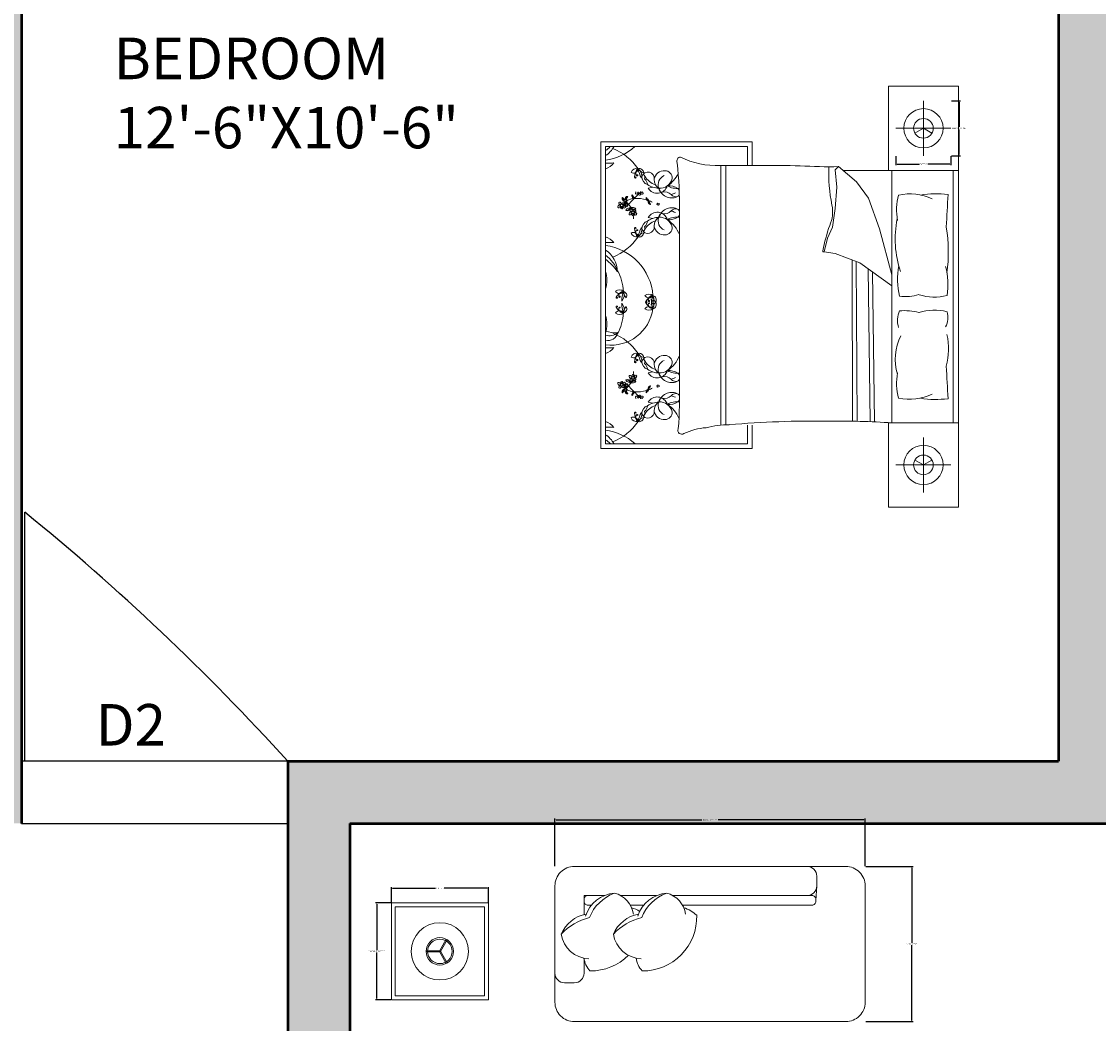
# Model space of a CAD drawing. Units: inches. Extents: x -12 to 604, y -566 to 58.
# Tile 9 of 12: x 280 to 436, y -219 to -74. Entities that reach past the tile are written whole.
import ezdxf

# ---------------------------------------------------------------- set-up
doc = ezdxf.new("R2010")
doc.units = ezdxf.units.IN
doc.header["$MEASUREMENT"] = 0
for name, color, linetype, lineweight in [('A-ANNO-DIMS', 2, 'Continuous', 18), ('A-ANNO-TEXT', 7, 'Continuous', 18), ('A-AREA-IDEN', 7, 'Continuous', 18), ('A-DOOR', 4, 'Continuous', 25), ('A-FURN', 8, 'Continuous', 18), ('A-WALL', 7, 'Continuous', 50), ('A-WALL-PATT', 18, 'Continuous', 13)]:
    doc.layers.add(name, color=color, linetype=linetype, lineweight=lineweight)
doc.styles.get("Standard").update_dxf_attribs({"font": 'arial.ttf'})
doc.dimstyles.get("Standard").update_dxf_attribs({"dimtxt": 0.18, "dimasz": 0.18, "dimexe": 0.18, "dimexo": 0.0625, "dimgap": 0.09, "dimtad": 0, "dimtih": 1, "dimtoh": 1, "dimdec": 0, "dimzin": 0, "dimdsep": 46, "dimlunit": 3, "dimtxsty": 'Standard', "dimcen": 0.09, "dimadec": 0, "dimazin": 0, "dimtfac": 1, "dimtdec": 0, "dimtofl": 0, "dimtmove": 0, "dimatfit": 3, "dimfxl": 1, "dimtolj": 1, "dimtzin": 0, "dimarcsym": 0})

# ---------------------------------------------------------------- blocks, each defined once
blk = doc.blocks.new('DAY BED1')
at = {"color": 0}
blk.add_line((0.3, 0.25), (0.225, 0.2549), dxfattribs=at)
blk.add_lwpolyline([(-0.3, 0, -0.414214), (-0.4, 0.1), (-0.4, 0.1, 0.317837), (-0.4, 0.1, -0.414214), (-0.4, 0.1), (-0.4, 0.1, 1.186185), (-0.4, 0.1, -0.414214), (-0.4, 0.1), (-0.4, 1.5, -0.414214), (-0.3, 1.6), (0.3, 1.6, -0.414214), (0.4, 1.5), (0.4, 0.1, -0.414214), (0.3, 0)], format="xyb", close=True, dxfattribs=at)
for points in [[(-0.0725, 1.45), (-0.15, 1.45, -0.414214), (-0.2, 1.5), (-0.2, 1.55, -0.414214), (-0.15, 1.6)], [(-0.0756, 1.4249, -0.356772), (0.0505, 1.5682, -0.249542), (0.1543, 1.4384, 9.61688)], [(0.0505, 1.5682, -0.14773), (0.1364, 1.422, -0.213343), (0.2624, 1.2931, -0.178662)], [(-0.0725, 1.4501, 0.165541), (-0.1386, 1.4192, 0.200231), (-0.0581, 1.2207, 0.121523)], [(0.25, 1.3448), (0.25, 1.45), (0.1517, 1.45, -0.414214)], [(0.2, 1.4118), (0.2, 1.43, -0.414214), (0.22, 1.45), (0.23, 1.45, -0.414214), (0.25, 1.43)], [(0.1433, 1.4422, -0.306663), (0.2624, 1.2931, -0.30633), (0.1536, 1.1957, 0.872847)], [(0.25, 1.43), (0.25, 1.3448, -0.414214)], [(-0.0756, 1.1556, -0.356772), (0.0505, 1.2988, -0.249542), (0.1543, 1.169, 9.61688)], [(0.0505, 1.2988, -0.14773), (0.1364, 1.1527, -0.213343), (0.2624, 1.0238, -0.178662)], [(0.25, 1.2616), (0.25, 1.0755, -0.414214)], [(-0.0725, 1.1808, 0.165541), (-0.1386, 1.1498, 0.425989), (0.1479, 0.869, 0.121523), (0.1873, 0.9357, -7.115464)], [(0.1433, 1.1729, -0.306663), (0.2624, 1.0238, -0.30633), (0.1536, 0.9263, 0.872847)], [(0.1678, 1.1631, 0.071865), (0.1873, 1.205, -7.115464)], [(0.2, 1.1425), (0.2, 1.2113, -0.414214)], [(0.25, 0.9923), (0.25, 0.2749, -0.414214), (0.23, 0.2549), (0.22, 0.2549, -0.414214), (0.2, 0.2749), (0.2, 0.9419, -0.414214)], [(0.25, 0.3775), (0.25, 0.3, 0.414214), (0.3, 0.25), (0.35, 0.25, 0.414214), (0.4, 0.3)]]:
    blk.add_lwpolyline(points, format="xyb", dxfattribs=at)
for points in [[(0.25, 1.0755), (0.25, 1.2616)], [(0.25, 0.3775), (0.25, 0.9923)]]:
    blk.add_lwpolyline(points, dxfattribs=at)
blk = doc.blocks.new('SIDE-TABLE-WITH-LAMP')
for p, q in [((6.94, 7.06), (7.93, 8.77)), ((7.09, 6.97), (8.08, 8.68)), ((7.01, 7.1), (5.03, 7.1)), ((7.01, 6.92), (5.03, 6.92)), ((6.94, 6.97), (7.93, 5.26)), ((7.09, 7.06), (8.08, 5.34))]:
    blk.add_line(p, q)
at = {"ltscale": 0.03}
blk.add_lwpolyline([(14.03, 14.03), (14.03, 0), (0, 0), (0, 14.03)], close=True, dxfattribs=at)
blk.add_lwpolyline([(13.46, 0.56), (13.46, 13.46), (0.56, 13.46), (0.56, 0.56)], close=True)
for radius in [4.14, 1.98, 1.77]:
    blk.add_circle((7.01, 7.01), radius)
blk = doc.blocks.new('BEDSIDE-LAMP-144')
for p, q in [((3.98, 7.95), (3.98, 0)), ((0, 3.98), (7.95, 3.98))]:
    blk.add_line(p, q)
for points in [[(3.98, 3.98), (2.75, 4.69)], [(3.98, 3.98), (5.21, 4.69)]]:
    blk.add_lwpolyline(points)
for radius in [2.84, 1.42]:
    blk.add_circle((3.98, 3.98), radius)
blk = doc.blocks.new('*D23')
at = {"layer": 'A-ANNO-DIMS', "color": 0, "lineweight": -2, "transparency": 16777216}
for p, q in [((357.47, -196.01), (357.47, -189.16)), ((357.65, -189.34), (378.73, -189.34)), ((402.17, -189.34), (381.1, -189.34)), ((402.35, -196.01), (402.35, -189.16))]:
    blk.add_line(p, q, dxfattribs=at)
at = {"layer": 'A-ANNO-DIMS', "color": 0, "transparency": 16777216}
for points in [[(357.65, -189.31), (357.65, -189.37), (357.47, -189.34)], [(402.17, -189.31), (402.17, -189.37), (402.35, -189.34)]]:
    blk.add_solid(points, dxfattribs=at)
at = {"layer": 'Defpoints', "color": 0, "transparency": 16777216}
for p in [(357.47, -189.34), (357.47, -196.07), (402.35, -196.07)]:
    blk.add_point(p, dxfattribs=at)
at = {"layer": 'A-ANNO-DIMS', "color": 0, "transparency": 16777216, "insert": (379.91, -189.34), "char_height": 0.18, "attachment_point": 5}
blk.add_mtext('\\A1;DAYBED 3\'-9" TYP.', dxfattribs=at)
blk = doc.blocks.new('*D24')
at = {"layer": 'A-ANNO-DIMS', "color": 0, "lineweight": -2, "transparency": 16777216}
for p, q in [((402.42, -196.07), (409.27, -196.07)), ((409.09, -196.25), (409.09, -207.11)), ((409.09, -218.33), (409.09, -207.47)), ((402.42, -218.51), (409.27, -218.51))]:
    blk.add_line(p, q, dxfattribs=at)
at = {"layer": 'A-ANNO-DIMS', "color": 0, "transparency": 16777216}
for points in [[(409.06, -196.25), (409.12, -196.25), (409.09, -196.07)], [(409.06, -218.33), (409.12, -218.33), (409.09, -218.51)]]:
    blk.add_solid(points, dxfattribs=at)
at = {"layer": 'Defpoints', "color": 0, "transparency": 16777216}
for p in [(402.35, -196.07), (409.09, -196.07), (402.35, -218.51)]:
    blk.add_point(p, dxfattribs=at)
at = {"layer": 'A-ANNO-DIMS', "color": 0, "transparency": 16777216, "insert": (409.09, -207.29), "char_height": 0.18, "attachment_point": 5}
blk.add_mtext('\\A1;1\'-10 1/2" TYP.', dxfattribs=at)
blk = doc.blocks.new('*D31')
at = {"layer": 'A-ANNO-DIMS', "color": 0, "lineweight": -2, "transparency": 16777216}
for p, q in [((333.76, -201.33), (331.53, -201.33)), ((331.71, -201.51), (331.71, -208.17)), ((331.71, -215.18), (331.71, -208.53)), ((333.76, -215.36), (331.53, -215.36))]:
    blk.add_line(p, q, dxfattribs=at)
at = {"layer": 'A-ANNO-DIMS', "color": 0, "transparency": 16777216}
for points in [[(331.68, -201.51), (331.74, -201.51), (331.71, -201.33)], [(331.68, -215.18), (331.74, -215.18), (331.71, -215.36)]]:
    blk.add_solid(points, dxfattribs=at)
at = {"layer": 'Defpoints', "color": 0, "transparency": 16777216}
for p in [(331.71, -201.33), (333.82, -201.33), (333.82, -215.36)]:
    blk.add_point(p, dxfattribs=at)
at = {"layer": 'A-ANNO-DIMS', "color": 0, "transparency": 16777216, "insert": (331.71, -208.35), "char_height": 0.18, "attachment_point": 5}
blk.add_mtext('\\A1;END TABLE 1\'-2" TYP.', dxfattribs=at)
blk = doc.blocks.new('*D32')
at = {"layer": 'A-ANNO-DIMS', "color": 0, "lineweight": -2, "transparency": 16777216}
for p, q in [((333.82, -201.27), (333.82, -199.05)), ((334, -199.23), (340.2, -199.23)), ((347.66, -199.23), (341.46, -199.23)), ((347.84, -201.27), (347.84, -199.05))]:
    blk.add_line(p, q, dxfattribs=at)
at = {"layer": 'A-ANNO-DIMS', "color": 0, "transparency": 16777216}
for points in [[(334, -199.2), (334, -199.26), (333.82, -199.23)], [(347.66, -199.2), (347.66, -199.26), (347.84, -199.23)]]:
    blk.add_solid(points, dxfattribs=at)
at = {"layer": 'Defpoints', "color": 0, "transparency": 16777216}
for p in [(347.84, -199.23), (333.82, -201.33), (347.84, -201.33)]:
    blk.add_point(p, dxfattribs=at)
at = {"layer": 'A-ANNO-DIMS', "color": 0, "transparency": 16777216, "insert": (340.83, -199.23), "char_height": 0.18, "attachment_point": 5}
blk.add_mtext('\\A1;1\'-2" TYP.', dxfattribs=at)
blk = doc.blocks.new('*D41')
at = {"layer": 'A-ANNO-DIMS', "color": 0, "lineweight": -2, "transparency": 16777216}
for p, q in [((414.81, -85.35), (416.12, -85.35)), ((415.94, -85.53), (415.94, -89.14)), ((415.94, -93.12), (415.94, -89.51)), ((414.81, -93.3), (416.12, -93.3))]:
    blk.add_line(p, q, dxfattribs=at)
at = {"layer": 'A-ANNO-DIMS', "color": 0, "transparency": 16777216}
for points in [[(415.91, -85.53), (415.97, -85.53), (415.94, -85.35)], [(415.91, -93.12), (415.97, -93.12), (415.94, -93.3)]]:
    blk.add_solid(points, dxfattribs=at)
at = {"layer": 'Defpoints', "color": 0, "transparency": 16777216}
for p in [(414.75, -85.35), (414.75, -93.3), (415.94, -93.3)]:
    blk.add_point(p, dxfattribs=at)
at = {"layer": 'A-ANNO-DIMS', "color": 0, "transparency": 16777216, "insert": (415.94, -89.33), "char_height": 0.18, "attachment_point": 5}
blk.add_mtext('\\A1;LAMP C 0\'-8" TYP.', dxfattribs=at)
blk = doc.blocks.new('*D42')
at = {"layer": 'A-ANNO-DIMS', "color": 0, "lineweight": -2, "transparency": 16777216}
for p, q in [((406.79, -93.37), (406.79, -94.68)), ((414.75, -93.37), (414.75, -94.68)), ((406.97, -94.5), (410.13, -94.5)), ((414.57, -94.5), (411.41, -94.5))]:
    blk.add_line(p, q, dxfattribs=at)
at = {"layer": 'A-ANNO-DIMS', "color": 0, "transparency": 16777216}
for points in [[(406.97, -94.47), (406.97, -94.53), (406.79, -94.5)], [(414.57, -94.47), (414.57, -94.53), (414.75, -94.5)]]:
    blk.add_solid(points, dxfattribs=at)
at = {"layer": 'Defpoints', "color": 0, "transparency": 16777216}
for p in [(406.79, -93.3), (414.75, -93.3), (406.79, -94.5)]:
    blk.add_point(p, dxfattribs=at)
at = {"layer": 'A-ANNO-DIMS', "color": 0, "transparency": 16777216, "insert": (410.77, -94.5), "char_height": 0.18, "attachment_point": 5}
blk.add_mtext('\\A1;0\'-8" TYP.', dxfattribs=at)

msp = doc.modelspace()

# ---------------------------------------------------------------- hatches: boundary and pattern name
at = {"layer": 'A-WALL-PATT'}
h = msp.add_hatch(color=256, dxfattribs=at)
h.dxf.hatch_style = 1
h.paths.add_polyline_path([(169.32, 11.14), (169.32, 17.14), (160.32, 17.14), (160.32, 11.14), (118.32, 11.14), (118.32, 6.64), (118.32, 2.14), (127.32, 2.14), (169.32, 2.14)])
h.paths.add_polyline_path([(127.32, -13.61), (118.32, -13.61), (118.32, -29.36), (34.82, -29.36), (24.32, -29.36), (24.32, -38.36), (39.32, -38.36), (118.32, -38.36), (118.32, -126.86), (127.32, -126.86), (127.32, -117.86)])
h.paths.add_polyline_path([(82.32, -92.36), (39.32, -92.36), (39.32, -56.22), (30.32, -56.22), (24.32, -56.22), (24.32, -65.22), (30.32, -65.22), (30.32, -113.36), (24.32, -113.36), (24.32, -122.36), (39.32, -122.36), (39.32, -101.36), (82.32, -101.36), (82.32, -96.86)], flags=17)
h.paths.add_polyline_path([(280.32, 11.14), (238.32, 11.14), (238.32, 17.14), (229.32, 17.14), (229.32, 12.64), (229.32, 11.14), (229.32, 2.14), (271.32, 2.14), (271.32, -117.86), (163.32, -117.86), (163.32, -126.86), (271.32, -126.86), (271.32, -189.86), (280.32, -189.86), (280.32, -180.86)])
h.paths.add_polyline_path([(415.32, 17.14), (406.32, 17.14), (406.32, 11.14), (358.32, 11.14), (358.32, -21.86), (367.32, -21.86), (367.32, 2.14), (415.32, 2.14)], flags=17)
h.paths.add_polyline_path([(484.55, -45.86), (448.32, -45.86), (448.32, 2.14), (448.32, 17.14), (439.32, 17.14), (439.32, 12.64), (439.32, 2.14), (439.32, -45.86), (367.32, -45.86), (358.32, -45.86), (358.32, -54.86), (430.32, -54.86), (430.32, -69.59), (430.32, -180.86), (318.82, -180.86), (318.82, -189.86), (318.82, -331.86), (327.82, -331.86), (327.82, -189.86), (439.32, -189.86), (439.32, -180.86), (439.32, -54.86), (483.5, -54.86), (484.55, -54.86)])
h.paths.add_polyline_path([(529.32, 11.14), (481.32, 11.14), (481.32, 17.14), (472.32, 17.14), (472.32, 12.64), (472.32, 2.14), (520.32, 2.14), (520.32, -21.86), (529.32, -21.86)])
h.paths.add_polyline_path([(598.32, -45.86), (582.42, -45.86), (582.42, -50.36), (582.42, -54.86), (589.32, -54.86), (589.32, -99.86), (598.32, -99.86), (604.32, -99.86), (604.32, -90.86), (598.32, -90.86)])
h.paths.add_polyline_path([(598.32, -168.86), (604.32, -168.86), (604.32, -159.86), (589.32, -159.86), (589.32, -180.86), (477.32, -180.86), (477.32, -189.86), (477.32, -259.86), (486.32, -259.86), (486.32, -189.86), (589.32, -189.86), (589.32, -204.86), (598.32, -204.86), (604.32, -204.86), (604.32, -195.86), (598.32, -195.86)])
h.paths.add_polyline_path([(598.32, -244.86), (604.32, -244.86), (604.32, -235.86), (598.32, -235.86), (589.32, -235.86), (589.32, -250.86), (522.32, -250.86), (522.32, -259.86), (589.32, -259.86), (589.32, -274.86), (598.32, -274.86), (604.32, -274.86), (604.32, -265.86), (598.32, -265.86)])
h.paths.add_polyline_path([(598.32, -333.28), (604.32, -333.28), (604.32, -324.28), (598.32, -324.28), (598.32, -321.87), (598.32, -318.28), (604.32, -318.28), (604.32, -309.28), (598.32, -309.28), (589.32, -309.28), (589.32, -341.95), (589.38, -341.95), (589.38, -363.16), (589.32, -381.86), (565.32, -381.86), (565.32, -390.86), (589.32, -390.86), (589.32, -450.86), (598.32, -450.86), (604.32, -450.86), (604.32, -441.86), (598.32, -441.86), (598.32, -390.86), (604.32, -390.86), (604.32, -381.86), (598.32, -381.86)])
h.paths.add_polyline_path([(541.32, -345.86), (424.32, -345.86), (424.32, -354.86), (532.32, -354.86), (532.32, -474.86), (463.39, -474.86), (463.39, -483.86), (553.32, -483.86), (553.32, -474.86), (541.32, -474.86), (541.32, -390.86), (541.32, -381.86)])
h.paths.add_polyline_path([(604.32, -474.86), (589.32, -474.86), (553.32, -474.86), (553.32, -483.86), (598.32, -483.86), (604.32, -483.86)])
h.paths.add_polyline_path([(388.32, -483.86), (388.32, -474.86), (388.32, -460.13), (388.32, -333.86), (388.32, -322.86), (379.32, -322.86), (379.32, -331.86), (379.32, -333.86), (379.32, -474.86), (379.32, -520.86), (344.32, -520.86), (344.32, -529.86), (379.32, -529.86), (388.32, -529.86)])
h.paths.add_polyline_path([(284.32, -520.86), (249.32, -520.86), (249.32, -474.86), (249.32, -368.36), (240.32, -368.36), (240.32, -474.86), (238.52, -474.86), (238.52, -483.86), (240.32, -483.86), (240.32, -529.86), (249.32, -529.86), (284.32, -529.86)])
h.paths.add_polyline_path([(178.82, -474.86), (158.91, -474.86), (158.91, -483.86), (162.32, -483.86), (178.82, -483.86)])
h.paths.add_polyline_path([(84.32, -474.86), (84.32, -366.86), (75.32, -366.86), (75.32, -474.86), (39.32, -474.86), (39.32, -453.86), (24.32, -453.86), (24.32, -462.86), (30.32, -462.86), (30.32, -483.86), (84.32, -483.86)])
h.paths.add_polyline_path([(39.32, -342.86), (75.32, -342.86), (84.32, -342.86), (179.67, -342.86), (179.67, -333.86), (39.32, -333.86), (39.32, -318.86), (24.32, -318.86), (24.32, -327.86), (30.32, -327.86), (30.32, -432.86), (24.32, -432.86), (24.32, -441.86), (30.32, -441.86), (39.32, -441.86)])
h.paths.add_polyline_path([(249.32, -252.86), (115.32, -252.86), (115.32, -225.86), (106.32, -225.86), (106.32, -252.86), (39.32, -252.86), (39.32, -237.86), (24.32, -237.86), (24.32, -246.86), (30.32, -246.86), (30.32, -267.86), (24.32, -267.86), (24.32, -276.86), (39.32, -276.86), (39.32, -261.86), (240.32, -261.86), (240.32, -331.86), (249.32, -331.86), (266.82, -331.86), (266.82, -322.86), (249.32, -322.86)])
h.paths.add_polyline_path([(127.32, -180.86), (39.32, -180.86), (24.32, -180.86), (24.32, -189.86), (39.32, -189.86), (127.32, -189.86)])
h.paths.add_polyline_path([(39.32, -159.86), (24.32, -159.86), (24.32, -168.86), (30.32, -168.86), (30.32, -180.86), (39.32, -180.86)])
h.paths.add_polyline_path([(470.51, -17.27), (512.48, -17.27), (512.48, 5.12), (470.51, 5.12)], flags=9)
h.paths.add_polyline_path([(484.21, -244.26), (526.45, -244.26), (526.45, -221.87), (484.21, -221.87)], flags=24)
h.paths.add_polyline_path([(36.91, -442.88), (83.54, -442.88), (83.54, -420.5), (36.91, -420.5)], flags=25)

# ---------------------------------------------------------------- linework, layer by layer
at = {"layer": 'A-DOOR'}
for p, q in [((280.8, -180.86), (280.8, -144.86)), ((318.82, -180.86), (280.32, -180.86)), ((280.32, -180.86), (280.32, -189.86)), ((318.82, -189.86), (318.82, -180.86)), ((280.32, -189.86), (318.82, -189.86))]:
    msp.add_line(p, q, dxfattribs=at)
msp.add_arc((63.22, -412.75), 345.12, 42.2146, 50.9159, dxfattribs=at)
at = {"layer": 'A-FURN'}
for p, q in [((415.84, -83.24), (415.84, -144.1)), ((364.09, -91.27), (386.01, -91.27)), ((364.09, -135.64), (364.09, -91.27)), ((386.01, -91.27), (386.01, -94.72)), ((364.79, -91.98), (364.79, -134.94)), ((385.3, -91.98), (364.79, -91.98)), ((385.3, -94.72), (385.3, -91.98)), ((381.46, -132.26), (381.46, -94.71)), ((382.21, -132.2), (382.21, -94.71)), ((398.01, -95.36), (398.5, -94.87)), ((398.5, -94.87), (401.09, -97.09)), ((398.26, -97.83), (398.01, -95.36)), ((415.84, -95.41), (399.14, -95.41)), ((406.22, -95.41), (406.22, -131.93)), ((415.06, -131.93), (415.06, -95.41)), ((370.96, -97.98), (371.65, -97.84)), ((398.01, -100.91), (398.26, -97.83)), ((401.09, -97.09), (402.81, -99.43)), ((402.81, -99.43), (404.42, -103.87)), ((397.64, -103.62), (398.01, -100.91)), ((370.96, -102.23), (371.65, -102.36)), ((375.48, -126.02), (375.48, -101.32)), ((396.9, -105.22), (397.64, -103.62)), ((404.42, -103.87), (406.22, -110.5)), ((396.41, -107.19), (396.9, -105.22)), ((398.01, -107.44), (396.41, -107.19)), ((401.58, -108.8), (398.01, -107.44)), ((400.53, -131.71), (400.44, -108.36)), ((401.16, -131.71), (401.06, -108.6)), ((406.22, -112.13), (401.58, -108.8)), ((403.07, -131.74), (402.76, -109.64)), ((403.7, -131.76), (403.39, -110.1)), ((370.96, -124.69), (371.65, -124.55)), ((370.96, -128.94), (371.65, -129.07)), ((385.3, -134.94), (385.3, -132.25)), ((386.01, -132.27), (386.01, -135.64)), ((364.79, -134.94), (385.3, -134.94)), ((386.01, -135.64), (364.09, -135.64))]:
    msp.add_line(p, q, dxfattribs=at)
for points in [[(405.7, -95.41), (405.7, -83.24), (415.84, -83.24)], [(415.84, -131.93), (405.7, -131.93), (405.7, -144.1), (415.84, -144.1)]]:
    msp.add_lwpolyline(points, dxfattribs=at)
for points in [[(392.93, -94.74, 0.001242), (381.38, -94.71, -0.127202), (375.63, -93.49)], [(414.33, -98.91, 0.074897), (410.35, -98.98, -0.472817)], [(410.13, -113.39, 0.14099), (414.18, -113.51, 0.235245)], [(410.13, -115.98, -0.14099), (414.18, -115.86, -0.235245)], [(414.33, -128.43, -0.074897), (410.35, -128.36, 0.472817)], [(382.69, -132.19, 0.056112), (379.34, -132.63, 0.095341), (376.12, -133.48)]]:
    msp.add_lwpolyline(points, format="xyb", dxfattribs=at)
for centre in [(367.12, -100.48), (368.76, -101.49), (368.76, -125.42), (367.12, -126.44)]:
    msp.add_circle(centre, 0.155, dxfattribs=at)
for centre, radius, start, end in [((361.94, -88.66), 4.83, 306.3036, 316.4814), ((362.66, -90.05), 3.87, 303.4617, 330.1116), ((363.72, -86.06), 7.95, 277.745, 311.8856), ((362.94, -99.66), 7.95, 34.3865, 68.5908), ((363.55, -92.22), 3.23, 292.5547, 318.9546), ((365.29, -83.37), 11, 267.4081, 273.6519), ((375.67, -94.05), 0.562, 93.98, 207.3412), ((312.13, -100.59), 63.35, 359.3433, 5.6887), ((396.99, -39.07), 55.82, 265.8294, 271.553), ((420.05, -95.91), 22.97, 177.4519, 191.3392), ((369.31, -96.03), 0.881, 77.7115, 159.0387), ((368.83, -95.15), 0.664, 238.4633, 358.2869), ((371.01, -96.49), 2.01, 138.8402, 177.9352), ((369.1, -96.43), 0.0987, 177.9352, 11.4834), ((369.15, -96.42), 0.0479, 11.4834, 127.9409), ((369.8, -95.75), 0.65, 117.6827, 223.7762), ((369.39, -96.14), 0.086, 223.7762, 159.7183), ((369.65, -95.81), 0.659, 2.9516, 103.728), ((374.92, -93.97), 5.56, 192.5173, 207.1824), ((368.76, -96.19), 1.26, 345.4653, 54.2343), ((370.65, -94.46), 1.36, 211.3827, 255.2969), ((370.91, -96.58), 0.913, 350.264, 160.8688), ((371.19, -96.37), 1.14, 175.969, 254.3045), ((369.92, -96.4), 0.56, 333.9755, 53.2681), ((372.92, -94.77), 2.87, 211.2614, 251.7045), ((373.26, -96.92), 1.45, 84.9449, 172.8857), ((373.81, -97.49), 1.41, 111.5819, 201.4221), ((373.4, -96.5), 1.03, 354.4856, 91.0538), ((371.19, -93.82), 4.61, 303.6671, 333.2997), ((369.67, -97.59), 1.21, 6.1662, 51.5825), ((372.69, -94.75), 3.27, 236.2883, 266.5076), ((372.27, -97.22), 1.51, 209.9085, 343.1337), ((373.58, -96.67), 1.77, 182.3591, 234.0401), ((372.64, -96.18), 1.83, 265.2933, 346.921), ((372.91, -98.18), 0.378, 167.3041, 285.1471), ((373.93, -99.99), 2.35, 122.7011, 126.3445), ((374.37, -97.46), 1.94, 199.2822, 299.1751), ((375.03, -95.5), 2.52, 238.8218, 279.1554), ((373.93, -99.99), 2.35, 55.785, 94.7304), ((374.8, -98.63), 0.733, 30.0293, 52.325), ((367.35, -99.48), 0.173, 124.3538, 214.3923), ((367.6, -99.5), 0.403, 190.3057, 287.1958), ((367.72, -99.36), 0.468, 176.9701, 248.2913), ((371.06, -96.89), 4.53, 212.6784, 216.3746), ((367.56, -99.47), 0.179, 216.3746, 291.7548), ((367.99, -99.6), 0.403, 122.8155, 187.3992), ((367.68, -99.76), 0.135, 289.3605, 111.7548), ((367.78, -99.76), 0.135, 221.8703, 44.2646), ((368.17, -99.65), 0.468, 109.4799, 177.6828), ((367.92, -99.35), 0.173, 56.8636, 146.9021), ((368, -99.54), 0.179, 148.8844, 224.2646), ((371.73, -101.79), 4.53, 145.1882, 148.8844), ((369.15, -101.99), 2.53, 94.756, 119.2041), ((374.53, -105.62), 8.32, 132.2412, 142.1744), ((370.33, -99.01), 1.72, 178.3264, 187.1302), ((368.48, -99.24), 0.32, 11.3256, 64.4621), ((369.56, -98.78), 0.962, 190.2588, 210.656), ((368.92, -99.18), 0.292, 188.3432, 274.2869), ((369.17, -99.01), 0.51, 210.656, 242.6341), ((369.56, -98.58), 0.978, 218.2101, 226.3071), ((368.83, -99.4), 0.124, 325.7657, 67.4417), ((364.99, -95.25), 5.78, 313.1541, 322.0459), ((369.27, -104.5), 5.04, 73.5842, 93.8277), ((369.23, -98.72), 0.119, 142.4737, 265.053), ((369.39, -98.7), 0.256, 127.7621, 169.0403), ((369.26, -98.48), 0.36, 265.053, 338.3618), ((369.73, -98.98), 0.471, 113.4276, 137.6104), ((369.68, -98.49), 0.155, 183.2768, 356.7232), ((369.79, -98.77), 0.254, 139.7889, 227.6792), ((369.71, -98.86), 0.134, 227.6792, 350.3487), ((369.19, -98.77), 0.507, 353.0852, 15.7171), ((369.53, -98.83), 0.32, 350.3487, 43.6538), ((370.12, -98.5), 0.373, 198.7263, 262.5032), ((369.82, -98.67), 0.148, 1.1081, 91.8675), ((370.1, -98.75), 0.12, 255.2356, 54.9248), ((369.92, -98.7), 0.258, 11.5637, 52.6358), ((372.38, -99.37), 1.72, 178.3264, 187.1302), ((370.52, -99.61), 0.32, 11.3256, 64.4621), ((371.61, -99.15), 0.962, 190.2588, 210.656), ((370.96, -99.54), 0.292, 188.3432, 274.2869), ((371.22, -99.38), 0.51, 210.656, 242.6341), ((371.61, -98.94), 0.978, 218.2101, 226.3071), ((370.88, -99.76), 0.124, 325.7657, 67.4417), ((373.33, -99.75), 1.25, 41.5653, 105.1471), ((374.02, -97.16), 1.75, 277.436, 299.9149), ((374.95, -98.32), 0.911, 221.5653, 293.8354), ((374.8, -98.63), 0.733, 314.4517, 333.558), ((415.04, -101.08), 8.16, 165.1039, 191.0369), ((408.75, -106.66), 7.84, 65.1316, 101.7583), ((993.48, -132.45), 580.12, 176.68521, 177.14978), ((366.68, -100.71), 0.119, 142.4737, 265.053), ((366.84, -100.69), 0.256, 61.2196, 169.0403), ((366.7, -100.47), 0.36, 265.053, 338.3618), ((367.01, -100.16), 0.306, 157.4086, 261.4386), ((366.83, -100.15), 0.154, 58.0499, 135.6268), ((367.18, -100.97), 0.471, 113.4276, 137.6104), ((366.99, -100.25), 0.103, 172.906, 277.132), ((366.66, -100.44), 0.489, 14.7558, 58.0499), ((367.24, -100.76), 0.254, 139.7889, 227.6792), ((367.16, -100.85), 0.134, 227.6792, 350.3487), ((367.34, -100.31), 0.211, 36.1046, 181.4281), ((366.64, -100.76), 0.507, 353.0852, 15.7171), ((366.97, -100.82), 0.32, 350.3487, 43.6538), ((367.57, -100.49), 0.373, 198.7263, 262.5032), ((367.22, -100.14), 0.213, 270.0645, 331.1507), ((367.4, -100.19), 0.244, 221.8413, 265.7877), ((367.27, -100.66), 0.148, 1.1081, 91.8675), ((367.4, -100.28), 0.152, 263.7526, 41.7054), ((367.36, -100.69), 0.258, 11.5637, 86.365), ((369.15, -101.99), 2.53, 124.0033, 132.4917), ((367.55, -100.74), 0.12, 255.2356, 54.9248), ((366.55, -102.3), 2.7, 63.7819, 68.2913), ((367.99, -100.23), 0.429, 128.3208, 208.8162), ((368.07, -100.2), 0.513, 207.7043, 254.3516), ((368.39, -100.16), 0.706, 157.2305, 229.0635), ((368.15, -99.92), 0.416, 174.4544, 220.6188), ((367.73, -100.49), 0.706, 270.278, 342.111), ((368.2, -101.37), 0.5, 98.7227, 159.3375), ((367.95, -100.73), 0.513, 244.9899, 291.6373), ((365.79, -102.25), 3.03, 30.544, 49.818), ((367.46, -100.52), 0.5, 340.0041, 40.6188), ((368.07, -100.47), 0.416, 278.7227, 324.8872), ((367.99, -100.81), 0.429, 290.5253, 358.5375), ((368.64, -101.18), 0.306, 157.4086, 261.4386), ((368.47, -101.17), 0.154, 58.0499, 135.6268), ((368.83, -100.68), 0.429, 182.8499, 266.1226), ((368.66, -100.38), 0.416, 231.7607, 277.9252), ((368.99, -100.31), 0.706, 214.5369, 286.3699), ((368.29, -101.45), 0.489, 14.7558, 58.0499), ((365.79, -102.25), 3.03, 23.0501, 23.8477), ((368.79, -101.29), 0.5, 37.3105, 97.9252), ((368.97, -101.32), 0.211, 36.1046, 181.4281), ((368.85, -100.6), 0.513, 265.0106, 311.658), ((369.03, -101.3), 0.152, 263.7526, 41.7054), ((371.23, -99.99), 0.292, 147.5332, 233.4768), ((371.49, -99.84), 0.51, 179.1859, 211.164), ((371, -99.95), 0.124, 354.3784, 96.0543), ((369.27, -104.5), 5.04, 63.0032, 69.8941), ((371.88, -99.6), 0.962, 211.164, 231.5612), ((372.05, -98.82), 1.72, 234.6898, 243.4936), ((372.06, -99.7), 0.978, 195.5129, 203.6099), ((370.96, -100.34), 0.32, 357.3579, 50.4944), ((372.34, -100.28), 0.117, 12.7051, 190.4384), ((372.41, -100.26), 0.191, 190.4384, 10.4136), ((374.37, -102.75), 1.94, 60.8249, 160.7178), ((374.95, -101.89), 0.911, 66.1646, 138.4347), ((374.8, -101.58), 0.733, 23.229, 45.5483), ((392.68, -101.4), 4.95, 336.2616, 11.3392), ((368.31, -101.73), 0.119, 142.4737, 265.053), ((368.47, -101.7), 0.256, 61.2196, 169.0403), ((368.33, -101.49), 0.36, 265.053, 338.3618), ((368.81, -101.98), 0.471, 113.4276, 137.6104), ((368.63, -101.26), 0.103, 172.906, 277.132), ((368.87, -101.77), 0.254, 139.7889, 227.6792), ((368.79, -101.86), 0.134, 227.6792, 350.3487), ((368.27, -101.77), 0.507, 353.0852, 15.7171), ((365.79, -102.25), 3.03, 357.1071, 4.7585), ((368.61, -101.83), 0.32, 350.3487, 43.6538), ((368.85, -101.16), 0.213, 270.0645, 331.1507), ((369.03, -101.21), 0.244, 221.8413, 265.7877), ((369.2, -101.5), 0.373, 198.7263, 262.5032), ((368.9, -101.67), 0.148, 1.1081, 91.8675), ((369, -101.71), 0.258, 11.5637, 86.365), ((369.18, -101.75), 0.12, 255.2356, 54.9248), ((371.19, -103.84), 1.14, 105.6955, 184.031), ((369.67, -102.61), 1.21, 308.4175, 353.8338), ((372.92, -105.43), 2.87, 108.2955, 148.7386), ((372.69, -105.46), 3.27, 93.4924, 123.7117), ((372.27, -102.98), 1.51, 16.8663, 150.0915), ((373.58, -103.54), 1.77, 125.9599, 177.6409), ((373.81, -102.72), 1.41, 158.5779, 248.4181), ((372.64, -104.02), 1.83, 13.079, 94.7067), ((372.91, -102.03), 0.378, 74.8529, 192.6959), ((373.93, -100.22), 2.35, 233.6555, 237.2989), ((373.33, -100.46), 1.25, 254.8529, 318.4347), ((375.03, -104.7), 2.52, 79.7133, 121.1782), ((373.93, -100.22), 2.35, 265.2696, 304.215), ((371.19, -106.39), 4.61, 21.4941, 56.3329), ((374.02, -103.04), 1.75, 60.0851, 82.564), ((374.8, -101.58), 0.733, 307.675, 336.7144), ((420.83, -105.37), 14.15, 168.0397, 199.2615), ((369.1, -103.78), 0.0987, 348.5166, 182.0648), ((371.01, -103.71), 2.01, 182.0648, 221.1598), ((369.15, -103.79), 0.0479, 232.0591, 348.5166), ((369.8, -104.46), 0.65, 136.2238, 242.3173), ((369.42, -104.08), 0.0518, 200.2667, 136.2271), ((368.76, -104.02), 1.26, 305.7657, 14.5347), ((374.92, -106.24), 5.56, 152.8176, 167.4827), ((370.91, -103.62), 0.913, 199.1312, 9.736), ((369.92, -103.81), 0.56, 306.7319, 26.0245), ((373.26, -103.29), 1.45, 187.1143, 275.0551), ((373.4, -103.71), 1.03, 268.9462, 5.5144), ((419.41, -111.42), 23.6, 160.1194, 169.3383), ((392.3, -107.25), 22.07, 352.2196, 9.497), ((363.55, -107.99), 3.23, 41.0454, 67.4453), ((365.29, -116.84), 11, 86.3481, 92.5919), ((362.94, -100.55), 7.95, 291.4092, 325.6135), ((368.83, -105.06), 0.664, 1.7131, 121.5367), ((369.31, -104.17), 0.881, 200.9613, 282.2885), ((369.65, -104.4), 0.659, 256.272, 357.0484), ((370.65, -105.74), 1.36, 104.7031, 148.6173), ((363.72, -114.14), 7.95, 4.4623, 82.255), ((362.66, -110.16), 3.87, 1.272, 56.5383), ((396.36, -107.06), 0.147, 178.8623, 289.7536), ((361.94, -111.55), 4.83, 17.8504, 53.6964), ((360.58, -114.09), 7.18, 34.0123, 54.053), ((360.61, -111.31), 4.37, 343.5431, 17.0202), ((359.47, -113.54), 7.95, 4.4623, 27.4146), ((417.75, -111.1), 10.73, 169.8617, 193.6238), ((403.46, -111.91), 10.84, 351.5249, 13.96), ((358.36, -113.04), 6.46, 4.3787, 5.6357), ((353.93, -116.45), 11.55, 19.7217, 19.9028), ((366.8, -113.57), 0.881, 47.7873, 129.1145), ((366.82, -112.57), 0.664, 208.5391, 328.3627), ((368.04, -114.82), 2.01, 108.9159, 148.011), ((367.36, -113.57), 0.65, 87.7585, 193.852), ((366.81, -113.7), 0.086, 193.852, 129.9245), ((372.69, -114.58), 5.56, 162.593, 177.2582), ((366.24, -113.43), 1.26, 315.5411, 24.3101), ((368.74, -112.88), 1.36, 181.4585, 225.3727), ((367.2, -113.55), 0.659, 333.0274, 73.8037), ((371.05, -114.18), 0.881, 47.7873, 129.1145), ((371.08, -113.18), 0.664, 208.5391, 328.3627), ((372.3, -115.43), 2.01, 108.9159, 148.011), ((371.62, -114.17), 0.65, 87.7585, 193.852), ((370.5, -114.04), 1.26, 315.5411, 24.3101), ((376.95, -115.19), 5.56, 162.593, 177.2582), ((371.46, -114.16), 0.659, 333.0274, 73.8037), ((373, -113.49), 1.36, 181.4585, 225.3727), ((408.09, -106.21), 7.46, 264.0129, 285.8293), ((366.42, -113.81), 0.0987, 148.011, 341.5592), ((366.42, -115.14), 0.0987, 18.4408, 211.989), ((368.04, -114.13), 2.01, 211.989, 251.0841), ((366.47, -113.82), 0.0479, 341.5592, 98.0167), ((366.47, -115.12), 0.0479, 261.9833, 18.4408), ((367.36, -115.38), 0.65, 166.148, 272.2415), ((366.85, -115.24), 0.0518, 230.1909, 166.0209), ((372.69, -114.36), 5.56, 182.7418, 197.407), ((366.24, -115.51), 1.26, 335.6899, 44.4589), ((368.74, -116.06), 1.36, 134.6273, 178.5415), ((367.2, -115.4), 0.659, 286.1963, 26.9726), ((371.08, -115.77), 0.664, 31.6373, 151.4609), ((370.68, -114.41), 0.0987, 148.011, 341.5592), ((370.68, -114.53), 0.0987, 18.4408, 211.989), ((372.3, -113.52), 2.01, 211.989, 251.0841), ((370.72, -114.43), 0.0479, 341.5592, 98.0167), ((370.72, -114.51), 0.0479, 261.9833, 18.4408), ((371.62, -114.77), 0.65, 166.148, 272.2415), ((371.07, -114.31), 0.086, 193.852, 129.9245), ((371.1, -114.63), 0.0518, 230.1909, 166.0209), ((370.5, -114.9), 1.26, 335.6899, 44.4589), ((376.95, -113.76), 5.56, 182.7418, 197.407), ((371.46, -114.79), 0.659, 286.1963, 26.9726), ((373, -115.45), 1.36, 134.6273, 178.5415), ((365.56, -114.54), 6.15, 262.8636, 351.8197), ((360.61, -117.63), 4.37, 342.9798, 16.4569), ((358.36, -115.9), 6.46, 354.3643, 355.6213), ((353.93, -112.5), 11.55, 340.0972, 340.2783), ((366.82, -116.38), 0.664, 31.6373, 151.4609), ((366.8, -115.38), 0.881, 230.8855, 312.2127), ((359.47, -115.41), 7.95, 332.5854, 355.5377), ((371.05, -114.77), 0.881, 230.8855, 312.2127), ((410.24, -117.1), 3.23, 155.0183, 198.5407), ((408.09, -123.16), 7.46, 74.1707, 95.9871), ((411.29, -116.7), 3.01, 333.3437, 16.1026), ((366.12, -115.34), 3.56, 248.117, 276.6195), ((365.13, -118.6), 1.43, 256.3898, 349.0739), ((365.32, -117.53), 1.8, 252.8609, 311.9049), ((362.94, -126.37), 7.95, 34.3865, 68.5908), ((414.44, -122.74), 7.75, 153.8761, 196.1746), ((403.68, -121.21), 10.7, 346.3427, 11.1841), ((365.29, -110.08), 11, 267.4081, 273.6519), ((363.55, -118.93), 3.23, 292.5547, 318.9546), ((369.31, -122.74), 0.881, 77.7115, 159.0387), ((368.83, -121.86), 0.664, 238.4633, 358.2869), ((371.01, -123.2), 2.01, 138.8402, 177.9352), ((369.8, -122.46), 0.65, 117.6827, 223.7762), ((369.39, -122.85), 0.086, 223.7762, 159.7183), ((369.65, -122.52), 0.659, 2.9516, 103.728), ((370.65, -121.17), 1.36, 211.3827, 255.2969), ((368.76, -122.9), 1.26, 345.4653, 54.2343), ((374.92, -120.68), 5.56, 192.5173, 207.1824), ((370.91, -123.29), 0.913, 350.264, 160.8688), ((371.19, -123.08), 1.14, 175.969, 254.3045), ((369.92, -123.11), 0.56, 333.9755, 53.2681), ((372.92, -121.48), 2.87, 211.2614, 251.7045), ((373.26, -123.63), 1.45, 84.9449, 172.8857), ((373.81, -124.2), 1.41, 111.5819, 201.4221), ((373.4, -123.21), 1.03, 354.4856, 91.0538), ((371.19, -120.52), 4.61, 303.6671, 338.5059), ((365.79, -124.67), 3.03, 355.2415, 2.8929), ((369.1, -123.13), 0.0987, 177.9352, 11.4834), ((369.15, -123.12), 0.0479, 11.4834, 127.9409), ((369.67, -124.3), 1.21, 6.1662, 51.5825), ((372.69, -121.46), 3.27, 236.2883, 266.5076), ((372.27, -123.93), 1.51, 209.9085, 343.1337), ((373.58, -123.38), 1.77, 182.3591, 234.0401), ((372.64, -122.89), 1.83, 265.2933, 346.921), ((375.03, -122.21), 2.52, 238.8218, 280.2867), ((373.93, -126.7), 2.35, 55.785, 94.7304), ((993.48, -94.89), 580.12, 182.85022, 183.31479), ((366.68, -126.2), 0.119, 94.947, 217.5263), ((366.7, -126.44), 0.36, 21.6382, 94.947), ((367.24, -126.16), 0.254, 132.3208, 220.2111), ((367.16, -126.07), 0.134, 9.6513, 132.3208), ((366.64, -126.16), 0.507, 344.2829, 6.9148), ((366.97, -126.1), 0.32, 316.3462, 9.6513), ((367.57, -126.43), 0.373, 97.4968, 161.2737), ((367.55, -126.18), 0.12, 305.0752, 104.7644), ((367.95, -126.19), 0.513, 68.3627, 115.0101), ((367.73, -126.43), 0.706, 17.889, 89.722), ((368.2, -125.54), 0.5, 200.6625, 261.2773), ((368.07, -126.45), 0.416, 35.1128, 81.2773), ((367.99, -126.11), 0.429, 1.4625, 69.4747), ((368.31, -125.19), 0.119, 94.947, 217.5263), ((368.47, -125.21), 0.256, 190.9597, 298.7804), ((368.33, -125.43), 0.36, 21.6382, 94.947), ((368.64, -125.74), 0.306, 98.5614, 202.5914), ((368.47, -125.75), 0.154, 224.3732, 301.9501), ((368.83, -126.23), 0.429, 93.8774, 177.1501), ((368.99, -126.61), 0.706, 73.6301, 145.4631), ((368.66, -126.54), 0.416, 82.0748, 128.2393), ((368.81, -124.94), 0.471, 222.3896, 246.5724), ((368.63, -125.65), 0.103, 82.868, 187.094), ((368.29, -125.46), 0.489, 301.9501, 345.2442), ((365.79, -124.67), 3.03, 336.1523, 336.9499), ((368.87, -125.14), 0.254, 132.3208, 220.2111), ((368.79, -125.05), 0.134, 9.6513, 132.3208), ((368.79, -125.63), 0.5, 262.0748, 322.6895), ((368.27, -125.15), 0.507, 344.2829, 6.9148), ((368.97, -125.59), 0.211, 178.5719, 323.8954), ((368.85, -126.32), 0.513, 48.342, 94.9894), ((368.61, -125.09), 0.32, 316.3462, 9.6513), ((369.2, -125.42), 0.373, 97.4968, 161.2737), ((369.03, -125.71), 0.244, 94.2123, 138.1587), ((368.85, -125.76), 0.213, 28.8493, 89.9355), ((368.9, -125.24), 0.148, 268.1325, 358.8919), ((369, -125.21), 0.258, 273.635, 348.4363), ((369.03, -125.62), 0.152, 318.2946, 96.2474), ((369.18, -125.16), 0.12, 305.0752, 104.7644), ((372.91, -124.89), 0.378, 167.3041, 285.1471), ((373.93, -126.7), 2.35, 122.7011, 126.3445), ((374.37, -124.17), 1.94, 199.2822, 299.1751), ((373.33, -126.46), 1.25, 41.5653, 105.1471), ((374.02, -123.87), 1.75, 277.436, 299.9149), ((374.95, -125.03), 0.911, 221.5653, 293.8354), ((374.8, -125.34), 0.733, 23.2856, 52.325), ((316.29, -127.89), 59.22, 355.2402, 1.8035), ((374.8, -125.34), 0.733, 314.4517, 336.7144), ((415.04, -126.26), 8.16, 168.9631, 194.8961), ((366.84, -126.23), 0.256, 190.9597, 298.7804), ((367.01, -126.75), 0.306, 98.5614, 202.5914), ((366.83, -126.76), 0.154, 224.3732, 301.9501), ((367.18, -125.95), 0.471, 222.3896, 246.5724), ((366.99, -126.67), 0.103, 82.868, 187.094), ((366.66, -126.48), 0.489, 301.9501, 345.2442), ((367.34, -126.61), 0.211, 178.5719, 323.8954), ((367.35, -127.44), 0.173, 145.6077, 235.6462), ((367.6, -127.41), 0.403, 72.8042, 169.6943), ((367.4, -126.72), 0.244, 94.2123, 138.1587), ((367.22, -126.77), 0.213, 28.8493, 89.9355), ((367.72, -127.55), 0.468, 111.7087, 183.0299), ((371.06, -130.02), 4.53, 143.6254, 147.3216), ((367.27, -126.26), 0.148, 268.1325, 358.8919), ((367.36, -126.22), 0.258, 273.635, 348.4363), ((367.4, -126.63), 0.152, 318.2946, 96.2474), ((367.56, -127.45), 0.179, 68.2452, 143.6254), ((369.15, -124.93), 2.53, 227.5083, 235.9967), ((366.55, -124.61), 2.7, 291.7087, 296.2181), ((367.99, -126.69), 0.429, 151.1838, 231.6792), ((367.99, -127.32), 0.403, 172.6008, 237.1845), ((368.07, -126.72), 0.513, 105.6484, 152.2957), ((367.68, -127.15), 0.135, 248.2452, 70.6395), ((367.78, -127.15), 0.135, 315.7354, 138.1297), ((368.39, -126.76), 0.706, 130.9365, 202.7695), ((368.17, -127.27), 0.468, 182.3172, 250.5201), ((368.15, -126.99), 0.416, 139.3812, 185.5456), ((365.79, -124.67), 3.03, 310.182, 329.456), ((367.92, -127.56), 0.173, 213.0979, 303.1364), ((368, -127.37), 0.179, 135.7354, 211.1156), ((367.46, -126.4), 0.5, 319.3812, 19.9959), ((371.73, -125.12), 4.53, 211.1156, 214.8118), ((369.15, -124.93), 2.53, 240.7959, 265.244), ((374.53, -121.29), 8.32, 217.8256, 227.7588), ((369.56, -128.13), 0.962, 149.344, 169.7412), ((370.33, -127.91), 1.72, 172.8698, 181.6736), ((368.92, -127.74), 0.292, 85.7131, 171.6568), ((369.17, -127.9), 0.51, 117.3659, 149.344), ((369.56, -128.34), 0.978, 133.6929, 141.7899), ((368.83, -127.52), 0.124, 292.5583, 34.2343), ((369.27, -122.42), 5.04, 266.1723, 286.4158), ((364.99, -131.66), 5.78, 37.9541, 46.8459), ((371.61, -127.77), 0.962, 149.344, 169.7412), ((372.38, -127.55), 1.72, 172.8698, 181.6736), ((370.52, -127.31), 0.32, 295.5379, 348.6744), ((370.96, -127.38), 0.292, 85.7131, 171.6568), ((371.22, -127.54), 0.51, 117.3659, 149.344), ((371.61, -127.98), 0.978, 133.6929, 141.7899), ((370.88, -127.16), 0.124, 292.5583, 34.2343), ((371.23, -126.93), 0.292, 126.5232, 212.4668), ((371.49, -127.08), 0.51, 148.836, 180.8141), ((371, -126.96), 0.124, 263.9457, 5.6216), ((369.27, -122.42), 5.04, 290.1059, 296.9968), ((371.88, -127.31), 0.962, 128.4388, 148.836), ((372.05, -128.1), 1.72, 116.5064, 125.3102), ((372.06, -127.21), 0.978, 156.3901, 164.4871), ((370.96, -126.57), 0.32, 309.5056, 2.6421), ((372.41, -126.65), 0.191, 349.5864, 169.5616), ((372.34, -126.64), 0.117, 169.5616, 347.2949), ((374.37, -129.46), 1.94, 60.8249, 160.7178), ((374.95, -128.6), 0.911, 66.1646, 138.4347), ((368.48, -127.67), 0.32, 295.5379, 348.6744), ((369.23, -128.19), 0.119, 94.947, 217.5263), ((369.39, -128.22), 0.256, 190.9597, 232.2379), ((369.26, -128.43), 0.36, 21.6382, 94.947), ((369.73, -127.94), 0.471, 222.3896, 246.5724), ((369.68, -128.43), 0.155, 3.2768, 176.7232), ((369.79, -128.15), 0.254, 132.3208, 220.2111), ((369.71, -128.06), 0.134, 9.6513, 132.3208), ((369.19, -128.15), 0.507, 344.2829, 6.9148), ((369.53, -128.09), 0.32, 316.3462, 9.6513), ((370.12, -128.42), 0.373, 97.4968, 161.2737), ((369.82, -128.25), 0.148, 268.1325, 358.8919), ((370.1, -128.17), 0.12, 305.0752, 104.7644), ((369.92, -128.21), 0.258, 307.3642, 348.4363), ((372.69, -132.17), 3.27, 93.4924, 123.7117), ((372.27, -129.69), 1.51, 16.8663, 150.0915), ((373.58, -130.25), 1.77, 125.9599, 177.6409), ((373.81, -129.43), 1.41, 158.5779, 248.4181), ((372.64, -130.73), 1.83, 13.079, 94.7067), ((372.91, -128.74), 0.378, 74.8529, 192.6959), ((373.93, -126.93), 2.35, 233.6555, 237.2989), ((373.33, -127.17), 1.25, 254.8529, 318.4347), ((375.03, -131.41), 2.52, 79.249, 121.1782), ((373.93, -126.93), 2.35, 265.2696, 304.215), ((371.19, -133.1), 4.61, 23.6453, 56.3329), ((374.02, -129.75), 1.75, 60.0851, 82.564), ((374.8, -128.29), 0.733, 307.675, 342.5814), ((374.8, -128.29), 0.733, 16.6343, 45.5483), ((408.75, -120.68), 7.84, 258.2417, 294.8684), ((369.1, -130.49), 0.0987, 348.5166, 182.0648), ((371.01, -130.42), 2.01, 182.0648, 221.1598), ((369.15, -130.5), 0.0479, 232.0591, 348.5166), ((369.8, -131.17), 0.65, 136.2238, 242.3173), ((369.42, -130.79), 0.0518, 200.2667, 136.2271), ((374.92, -132.95), 5.56, 152.8176, 167.4827), ((368.76, -130.73), 1.26, 305.7657, 14.5347), ((371.19, -130.55), 1.14, 105.6955, 184.031), ((370.91, -130.33), 0.913, 199.1312, 9.736), ((369.92, -130.52), 0.56, 306.7319, 26.0245), ((369.67, -129.32), 1.21, 308.4175, 353.8338), ((372.92, -132.14), 2.87, 108.2955, 148.7386), ((373.26, -130), 1.45, 187.1143, 275.0551), ((373.4, -130.42), 1.03, 268.9462, 5.5144), ((363.55, -134.7), 3.23, 41.0454, 67.4453), ((362.94, -127.26), 7.95, 291.4092, 325.6135), ((368.83, -131.76), 0.664, 1.7131, 121.5367), ((369.31, -130.88), 0.881, 200.9613, 282.2885), ((370.65, -132.45), 1.36, 104.7031, 148.6173), ((369.65, -131.1), 0.659, 256.272, 357.0484), ((394.81, -274.31), 142.64, 89.1145, 94.8735), ((398.79, -241.02), 109.35, 86.1, 90.9282), ((365.29, -143.55), 11, 86.3481, 92.5919), ((363.72, -140.85), 7.95, 48.1144, 82.255), ((362.66, -136.87), 3.87, 29.8884, 56.5383), ((375.81, -133.02), 0.555, 156.5219, 303.8264), ((361.94, -138.26), 4.83, 43.5186, 53.6964)]:
    msp.add_arc(centre, radius, start, end, dxfattribs=at)
at = {"layer": 'A-WALL'}
for p, q in [((280.32, 11.14), (280.32, -189.86)), ((430.32, -54.86), (430.32, -180.86)), ((318.82, -180.86), (430.32, -180.86)), ((318.82, -180.86), (318.82, -331.86)), ((327.82, -189.86), (439.32, -189.86)), ((327.82, -189.86), (327.82, -331.86))]:
    msp.add_line(p, q, dxfattribs=at)

# ---------------------------------------------------------------- block references
at = {"layer": 'A-FURN', "rotation": 180}
msp.add_blockref('BEDSIDE-LAMP-144', (414.75, -85.35), dxfattribs=at)
at = {"layer": 'A-FURN'}
for name, p in [('BEDSIDE-LAMP-144', (406.79, -141.99)), ('SIDE-TABLE-WITH-LAMP', (333.82, -215.36))]:
    msp.add_blockref(name, p, dxfattribs=at)
at = {"layer": 'A-FURN', "ltscale": 0.03, "xscale": 28.05029504973475, "yscale": 28.05029504973475, "zscale": 28.05029504973475, "rotation": 90.00000000000006}
msp.add_blockref('DAY BED1', (402.35, -207.29), dxfattribs=at)

# ---------------------------------------------------------------- texts
at = {"layer": 'A-ANNO-TEXT', "insert": (291.04, -172.59), "char_height": 6, "attachment_point": 1}
msp.add_mtext('D2', dxfattribs=at)
at = {"layer": 'A-AREA-IDEN', "insert": (293.65, -76.23), "char_height": 6, "attachment_point": 1}
msp.add_mtext('BEDROOM\\P12\'-6"X10\'-6"', dxfattribs=at)

# ---------------------------------------------------------------- dimensions: what is measured, and where the dimension line sits
at = {"layer": 'A-ANNO-DIMS'}
for base, p1, p2, angle, text, picture, middle in [((415.9391, -93.3038), (414.7464, -85.3518), (414.7464, -93.3038), 270, 'LAMP C <> TYP.', '*D41', (415.9391, -89.3278)), ((406.79, -94.5), (414.75, -93.3), (406.79, -93.3), 180, '<> TYP.', '*D42', (410.77, -94.5)), ((357.47, -189.34), (402.35, -196.07), (357.47, -196.07), 180, 'DAYBED <> TYP.', '*D23', (379.91, -189.34)), ((409.09, -196.07), (402.35, -218.51), (402.35, -196.07), 90, '<> TYP.', '*D24', (409.09, -207.29)), ((331.71, -201.33), (333.82, -215.36), (333.82, -201.33), 90, 'END TABLE <> TYP.', '*D31', (331.71, -208.35))]:
    dim = msp.add_linear_dim(base=base, p1=p1, p2=p2, angle=angle, text=text, dimstyle='Standard', override={"dimdec": 1, "dimlfac": 1, "dimrnd": 0, "dimzin": 1, "dimdsep": 46, "dimlunit": 4, "dimfrac": 2}, dxfattribs=at)
    dim.commit()
    dim.dimension.update_dxf_attribs({"geometry": picture, "text_midpoint": middle})
dim = msp.add_linear_dim(base=(347.84, -199.23), p1=(333.82, -201.33), p2=(347.84, -201.33), text='<> TYP.', dimstyle='Standard', override={"dimdec": 1, "dimlfac": 1, "dimrnd": 0, "dimzin": 1, "dimdsep": 46, "dimlunit": 4, "dimfrac": 2}, dxfattribs=at)
dim.commit()
dim.dimension.update_dxf_attribs({"geometry": '*D32', "text_midpoint": (340.83, -199.23)})

doc.saveas('drawing.dxf')
